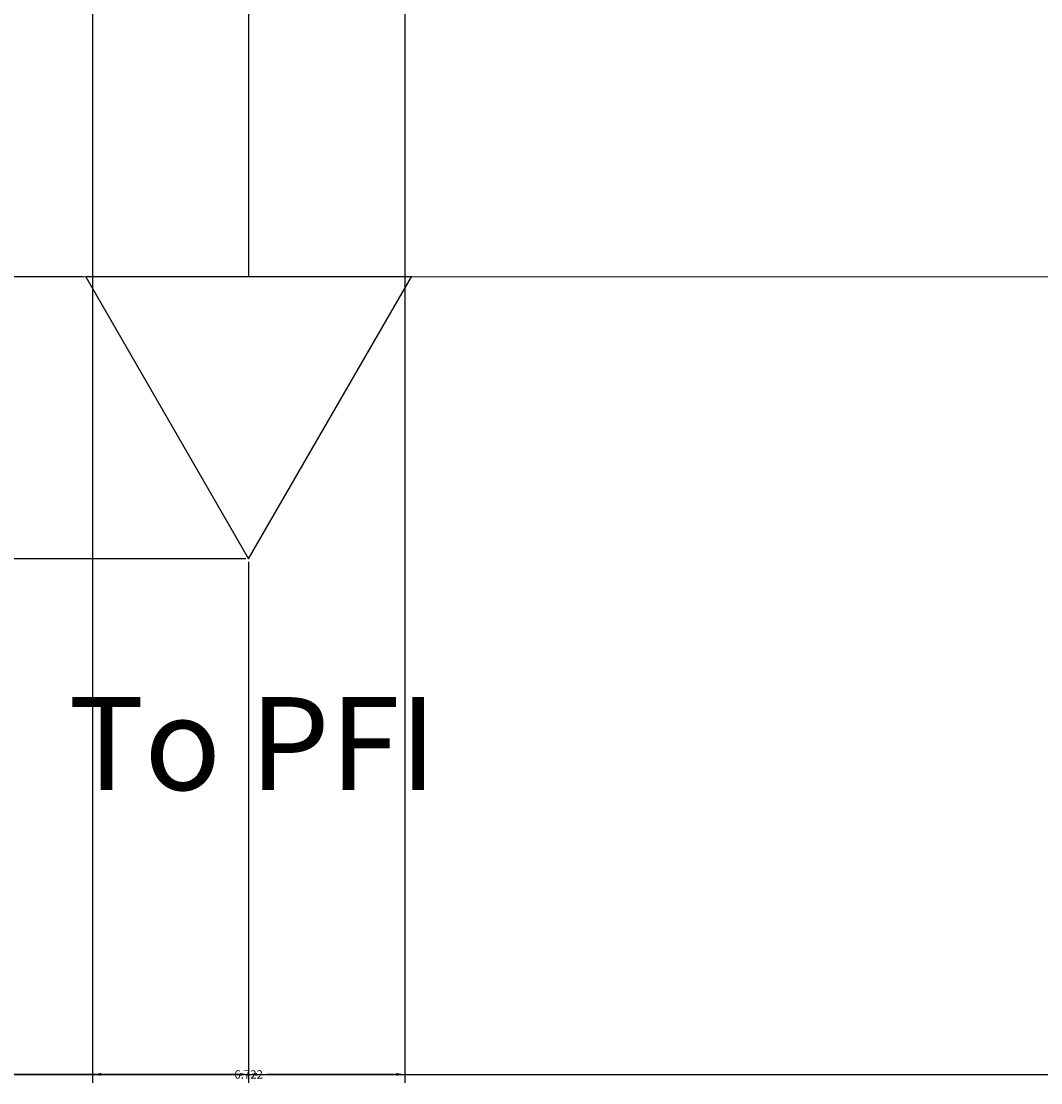
# Model space of a CAD drawing. Units: inches. Extents: x 412 to 584, y 208 to 437.
# Tile 2 of 28: x 450 to 472, y 208 to 231. Entities that reach past the tile are written whole.
import ezdxf

# ---------------------------------------------------------------- set-up
doc = ezdxf.new("R2010")
doc.units = ezdxf.units.IN
doc.header["$MEASUREMENT"] = 0
for name, color, linetype, lineweight in [('A-ANNO-DIMS', 2, 'Continuous', 18), ('E-ANNO-TEXT', 7, 'Continuous', 18), ('E-ENCL', 8, 'Continuous', 18), ('E-POWR-EQPM', 3, 'Continuous', 25)]:
    doc.layers.add(name, color=color, linetype=linetype, lineweight=lineweight)
doc.styles.get("Standard").update_dxf_attribs({"font": 'arial.ttf'})
doc.dimstyles.get("Standard").update_dxf_attribs({"dimtxt": 0.18, "dimasz": 0.18, "dimexe": 0.18, "dimexo": 0.0625, "dimgap": 0.09, "dimtad": 0, "dimtih": 1, "dimtoh": 1, "dimdec": 4, "dimzin": 0, "dimdsep": 46, "dimtxsty": 'Standard', "dimcen": 0.09, "dimadec": 0, "dimazin": 0, "dimtfac": 1, "dimtdec": 4, "dimtofl": 0, "dimtmove": 0, "dimatfit": 3, "dimfxl": 1, "dimtolj": 1, "dimtzin": 0, "dimarcsym": 0})

# ---------------------------------------------------------------- blocks, each defined once
blk = doc.blocks.new('*U3')
blk.add_line((-0.212, 0.212), (0.212, -0.212))
blk = doc.blocks.new('*U4')
at = {"color": 0, "linetype": 'ByBlock', "lineweight": -2, "transparency": 16777216}
for p, rotation in [((224.254, 56.203), 180), ((224.677, 56.203), 89.99999999999999), ((224.254, 55.78), 269.9999999999999)]:
    blk.add_blockref('*U3', p, dxfattribs=dict(at, rotation=rotation))
blk.add_blockref('*U3', (224.677, 55.78), dxfattribs=at)
blk = doc.blocks.new('*U7')
blk.add_line((-0.288, 0.288), (0.288, -0.288))
blk = doc.blocks.new('*U8')
at = {"color": 0, "linetype": 'ByBlock', "lineweight": -2, "transparency": 16777216}
for p, rotation in [((224.177, 56.28), 180), ((224.754, 56.28), 90), ((224.177, 55.703), 269.9999999999999)]:
    blk.add_blockref('*U7', p, dxfattribs=dict(at, rotation=rotation))
blk.add_blockref('*U7', (224.754, 55.703), dxfattribs=at)
blk = doc.blocks.new('MCCB-800A')
for q in [(1.94, 18.628), (3.361, 0)]:
    blk.add_line((3.361, 14.893), q)
blk.add_lwpolyline([(0, 20.016), (6.722, 20.016), (6.722, 12.209), (0, 12.209)], close=True)
blk.add_circle((3.361, 14.5), 0.393)
for name in ['*U8', '*U4']:
    blk.add_blockref(name, (-221.104, -36.809))
blk = doc.blocks.new('*D13')
at = {"layer": 'A-ANNO-DIMS', "color": 0, "lineweight": -2, "transparency": 16777216}
for p, q in [((423.556, 225.526), (423.556, 208.233)), ((572.394, 225.526), (572.394, 208.233)), ((423.736, 208.413), (497.52, 208.413)), ((572.214, 208.413), (498.43, 208.413))]:
    blk.add_line(p, q, dxfattribs=at)
at = {"layer": 'A-ANNO-DIMS', "color": 0, "transparency": 16777216}
for points in [[(423.736, 208.443), (423.736, 208.383), (423.556, 208.413)], [(572.214, 208.443), (572.214, 208.383), (572.394, 208.413)]]:
    blk.add_solid(points, dxfattribs=at)
at = {"layer": 'Defpoints', "color": 0, "transparency": 16777216}
for p in [(423.556, 225.588), (572.394, 225.588), (572.394, 208.413)]:
    blk.add_point(p, dxfattribs=at)
at = {"layer": 'A-ANNO-DIMS', "color": 0, "transparency": 16777216, "insert": (497.975, 208.413), "char_height": 0.18, "attachment_point": 5}
blk.add_mtext('\\A1;148.84', dxfattribs=at)
blk = doc.blocks.new('*D14')
at = {"layer": 'A-ANNO-DIMS', "color": 0, "lineweight": -2, "transparency": 16777216}
for p, q in [((423.556, 225.526), (423.556, 208.233)), ((454.644, 219.451), (454.644, 208.233)), ((423.736, 208.413), (438.706, 208.413)), ((454.464, 208.413), (439.494, 208.413))]:
    blk.add_line(p, q, dxfattribs=at)
at = {"layer": 'A-ANNO-DIMS', "color": 0, "transparency": 16777216}
for points in [[(423.736, 208.443), (423.736, 208.383), (423.556, 208.413)], [(454.464, 208.443), (454.464, 208.383), (454.644, 208.413)]]:
    blk.add_solid(points, dxfattribs=at)
at = {"layer": 'Defpoints', "color": 0, "transparency": 16777216}
for p in [(423.556, 225.588), (454.644, 219.513), (454.644, 208.413)]:
    blk.add_point(p, dxfattribs=at)
at = {"layer": 'A-ANNO-DIMS', "color": 0, "transparency": 16777216, "insert": (439.1, 208.413), "char_height": 0.18, "attachment_point": 5}
blk.add_mtext('\\A1;31.09', dxfattribs=at)
blk = doc.blocks.new('*D15')
at = {"layer": 'A-ANNO-DIMS', "color": 0, "lineweight": -2, "transparency": 16777216}
for p, q in [((454.644, 219.451), (454.644, 208.233)), ((499.288, 219.47), (499.288, 208.233)), ((454.824, 208.413), (476.569, 208.413)), ((499.108, 208.413), (477.363, 208.413))]:
    blk.add_line(p, q, dxfattribs=at)
at = {"layer": 'A-ANNO-DIMS', "color": 0, "transparency": 16777216}
for points in [[(454.824, 208.443), (454.824, 208.383), (454.644, 208.413)], [(499.108, 208.443), (499.108, 208.383), (499.288, 208.413)]]:
    blk.add_solid(points, dxfattribs=at)
at = {"layer": 'Defpoints', "color": 0, "transparency": 16777216}
for p in [(454.644, 219.513), (499.288, 219.533), (499.288, 208.413)]:
    blk.add_point(p, dxfattribs=at)
at = {"layer": 'A-ANNO-DIMS', "color": 0, "transparency": 16777216, "insert": (476.966, 208.413), "char_height": 0.18, "attachment_point": 5}
blk.add_mtext('\\A1;44.64', dxfattribs=at)
blk = doc.blocks.new('*D36')
at = {"layer": 'A-ANNO-DIMS', "color": 0, "lineweight": -2, "transparency": 16777216}
for p, q in [((451.283, 237.734), (451.283, 208.233)), ((458.005, 237.734), (458.005, 208.233)), ((451.463, 208.413), (454.251, 208.413)), ((457.825, 208.413), (455.037, 208.413))]:
    blk.add_line(p, q, dxfattribs=at)
at = {"layer": 'A-ANNO-DIMS', "color": 0, "transparency": 16777216}
for points in [[(451.463, 208.443), (451.463, 208.383), (451.283, 208.413)], [(457.825, 208.443), (457.825, 208.383), (458.005, 208.413)]]:
    blk.add_solid(points, dxfattribs=at)
at = {"layer": 'Defpoints', "color": 0, "transparency": 16777216}
for p in [(451.283, 237.797), (458.005, 237.797), (458.005, 208.413)]:
    blk.add_point(p, dxfattribs=at)
at = {"layer": 'A-ANNO-DIMS', "color": 0, "transparency": 16777216, "insert": (454.644, 208.413), "char_height": 0.18, "attachment_point": 5}
blk.add_mtext('\\A1;6.722', dxfattribs=at)
blk = doc.blocks.new('*D38')
at = {"layer": 'A-ANNO-DIMS', "color": 0, "lineweight": -2, "transparency": 16777216}
for p, q in [((451.074, 225.588), (412.276, 225.588)), ((412.456, 225.408), (412.456, 222.733)), ((412.456, 219.693), (412.456, 222.369)), ((454.582, 219.513), (412.276, 219.513))]:
    blk.add_line(p, q, dxfattribs=at)
at = {"layer": 'A-ANNO-DIMS', "color": 0, "transparency": 16777216}
for points in [[(412.426, 225.408), (412.486, 225.408), (412.456, 225.588)], [(412.426, 219.693), (412.486, 219.693), (412.456, 219.513)]]:
    blk.add_solid(points, dxfattribs=at)
at = {"layer": 'Defpoints', "color": 0, "transparency": 16777216}
for p in [(451.137, 225.588), (412.456, 219.513), (454.644, 219.513)]:
    blk.add_point(p, dxfattribs=at)
at = {"layer": 'A-ANNO-DIMS', "color": 0, "transparency": 16777216, "insert": (412.456, 222.551), "char_height": 0.18, "attachment_point": 5}
blk.add_mtext('\\A1;6.075', dxfattribs=at)

msp = doc.modelspace()

# ---------------------------------------------------------------- linework, layer by layer
at = {"layer": 'E-ENCL'}
msp.add_lwpolyline([(423.5562, 309.3773), (572.3937, 309.3773), (572.3937, 225.5881), (423.5562, 225.5881)], close=True, dxfattribs=at)
at = {"layer": 'E-POWR-EQPM'}
msp.add_lwpolyline([(454.6441, 219.5133), (458.1514, 225.5881), (451.1367, 225.5881)], close=True, dxfattribs=at)

# ---------------------------------------------------------------- block references
msp.add_blockref('MCCB-800A', (451.283, 225.588), dxfattribs=at)

# ---------------------------------------------------------------- texts
at = {"layer": 'E-ANNO-TEXT', "insert": (447.913, 216.537), "char_height": 2, "attachment_point": 1}
msp.add_mtext_dynamic_manual_height_columns('\\pxqc;{To PFI}', width=13.633448, gutter_width=1, heights=[2.9648], dxfattribs=at)

# ---------------------------------------------------------------- dimensions: what is measured, and where the dimension line sits
at = {"layer": 'A-ANNO-DIMS'}
for base, p1, p2, override, picture, middle in [((458.0051, 208.4133), (451.283, 237.797), (458.0051, 237.797), {"dimdec": 3, "dimlfac": 1, "dimrnd": 0, "dimzin": 0, "dimdsep": 46, "dimlunit": 2}, '*D36', (454.6441, 208.4133)), ((572.3937, 208.4133), (423.5562, 225.5881), (572.3937, 225.5881), {"dimdec": 2, "dimlfac": 1, "dimrnd": 0, "dimzin": 0, "dimdsep": 46, "dimlunit": 2}, '*D13', (497.975, 208.4133)), ((454.6441, 208.4133), (423.5562, 225.5881), (454.6441, 219.5133), {"dimdec": 2, "dimlfac": 1, "dimrnd": 0, "dimzin": 0, "dimdsep": 46, "dimlunit": 2}, '*D14', (439.1001, 208.4133)), ((499.2878, 208.4133), (454.6441, 219.5133), (499.2878, 219.5329), {"dimdec": 2, "dimlfac": 1, "dimrnd": 0, "dimzin": 0, "dimdsep": 46, "dimlunit": 2}, '*D15', (476.9659, 208.4133))]:
    dim = msp.add_linear_dim(base=base, p1=p1, p2=p2, dimstyle='Standard', override=override, dxfattribs=at)
    dim.commit()
    dim.dimension.update_dxf_attribs({"geometry": picture, "text_midpoint": middle})
dim = msp.add_linear_dim(base=(412.4562, 219.5133), p1=(451.1367, 225.5881), p2=(454.6441, 219.5133), angle=90, dimstyle='Standard', override={"dimdec": 3, "dimlfac": 1, "dimrnd": 0, "dimzin": 0, "dimdsep": 46, "dimlunit": 2}, dxfattribs=at)
dim.commit()
dim.dimension.update_dxf_attribs({"geometry": '*D38', "text_midpoint": (412.4562, 222.5507)})

doc.saveas('drawing.dxf')
